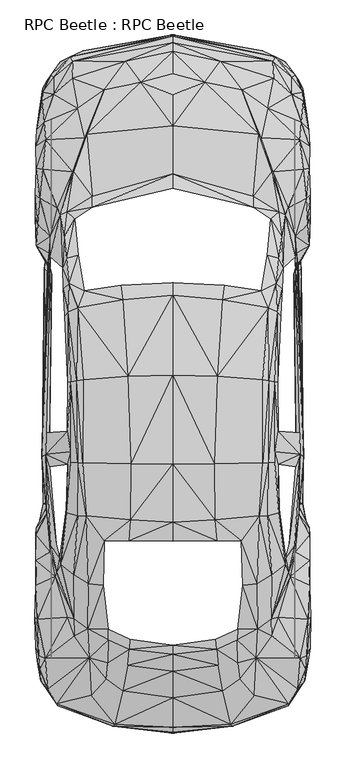
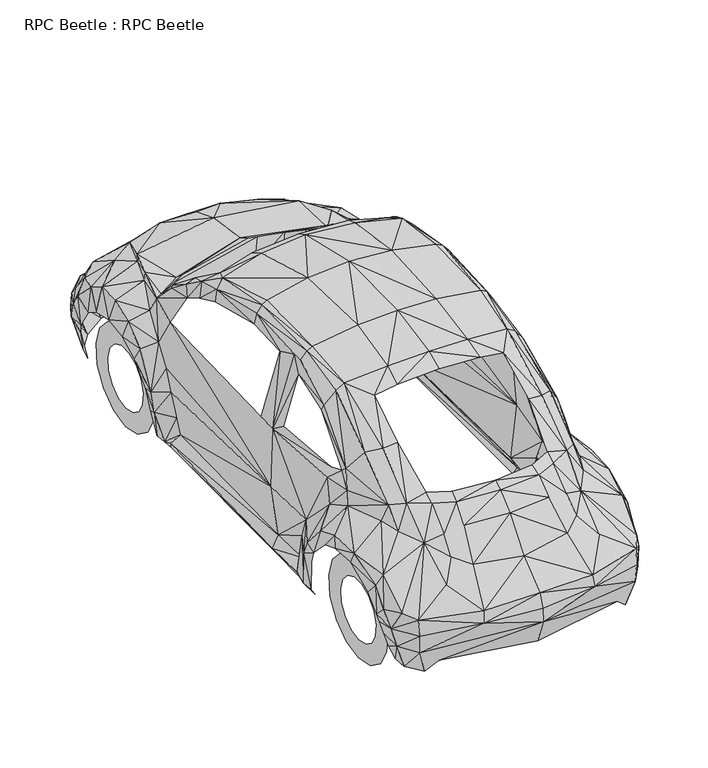
"""IFC4 building model written with IfcOpenShell, lengths in millimetres: proxy geometry, RPC Beetle : RPC Beetle."""

from ifc_helpers import new_model, si_unit, origin, place, context, project, spatial, triangles, source, transform, mapped, element, save


def rpc_beetle_rpc_beetle_31f8b51e(model_context):
    return source(origin(), model_context, "Body", "Tessellation", [
        triangles([(0.0, -748.5640469, 521.3894322), (0.0, -720.14536, 603.624202), (0.0, -696.6746996, 283.1362969), (0.0, -552.698168, 738.4051466), (0.0, -753.249444, 438.4540512), (0.0, -253.6666567, 1039.7136446), (0.0, -401.1024794, 921.3971746), (0.0, -304.8115909, 1012.258271), (0.0, 339.3169338, 1395.7139351), (0.0, 448.6129515, 1442.1297066), (0.0, 778.077507, 1504.0467121), (0.0, 1285.0167675, 1509.4764679), (0.0, 1741.0736687, 1402.3260315), (0.0, 2430.9612099, 967.1999022), (0.0, 3130.000518, 632.0428888), (0.0, 3001.4374352, 771.5092306), (0.0, 2704.2451103, 928.7536297), (0.0, 3164.1993027, 220.1684652), (0.0, 2883.1647125, 858.7358831), (0.0, 3222.5256844, 395.8040746), (0.0, 3178.9998528, 555.7633879), (0.0, 3213.9430687, 530.2784972), (-338.1784132, -715.5037828, 523.0096095), (-331.0409128, -702.1482754, 593.4652654), (-244.7338081, -218.0228295, 1034.0649342), (-248.9812959, -275.9549947, 1002.9312967), (-257.7389917, -368.17353, 911.8513184), (-249.0688632, 342.8199903, 1381.001025), (-285.238149, -511.5370176, 760.4306917), (-240.1360146, 460.0855433, 1426.5848705), (-236.4577871, 780.8799522, 1493.4060825), (-652.4921494, -590.2249108, 370.4943186), (-540.0870918, -593.333878, 283.4428189), (-181.240518, 2954.2772324, 806.3210592), (-253.1849819, 1278.5798058, 1496.1647804), (-379.8650402, -444.3655, 798.2639929), (-370.9321916, -353.3292326, 889.1688366), (-367.9983953, -222.2265337, 1003.4567734), (-368.3924847, -160.7037264, 1036.6922447), (-390.1553641, 342.863774, 1359.0192272), (-282.5670547, 1713.2680984, 1399.3047043), (-397.3366482, 87.4893818, 1215.3492176), (-463.1069432, -537.7663033, 704.8193333), (-271.4885704, 3072.331073, 662.6948696), (-475.7618394, -323.0714138, 849.8468182), (-463.7199872, 3085.9055351, 214.2570346), (-482.2425121, 95.7654028, 1203.3950054), (-485.0449937, -159.3024857, 1005.0769506), (-568.7247697, 3071.499147, 546.7429356), (-493.539933, 483.2496454, 1391.2913853), (-583.2625451, 3099.3922119, 522.0462599), (-510.267146, 3132.2774139, 369.399618), (-391.8631087, 2911.6272194, 782.7628315), (-656.3455479, -597.8441042, 480.0968946), (-660.2426937, -584.8389387, 576.2563957), (-562.2878443, -200.0695649, 879.7105476), (-560.0546594, -101.457906, 987.167506), (-512.4565836, 786.1783207, 1448.435281), (-541.7948364, 484.7822554, 1359.8511532), (-563.9956252, 148.5743069, 1172.305188), (-608.4846974, -561.2369273, 218.4607206), (-511.2742793, 1258.5246346, 1456.1858253), (-542.4078804, 784.6895308, 1430.657151), (-458.8594554, 2304.0621243, 949.0276829), (-601.0406751, -92.7440029, 893.1973698), (-503.7426533, 1765.2887604, 1320.9670441), (-546.0423243, 1253.0073841, 1441.5166626), (-603.011158, 501.1591264, 1278.5798058), (-580.1535416, 788.8932713, 1378.7239838), (-607.2148258, 519.8568223, 1235.1416142), (-601.2595934, 965.2732029, 1337.0374294), (-712.4823103, -503.0858256, 590.4876492), (-542.6706187, 1670.0487888, 1361.1648811), (-490.6061368, 2657.8732315, 893.5038918), (-599.6394161, 778.077507, 1307.3050873), (-598.0630589, 1243.7242298, 1343.7809132), (-639.5745512, 208.1266494, 1062.483621), (-680.4291796, -470.2006963, 218.6796571), (-538.4669146, 1966.7157097, 1180.581209), (-580.9855402, 1248.2344196, 1401.7567348), (-644.5226503, 243.2887836, 1028.2848364), (-502.3414307, 2635.8036484, 866.0047709), (-660.7243504, 162.2363182, 955.24569), (-690.2378105, -396.5922532, 226.8243271), (-559.1350934, 2175.0175301, 1011.1635704), (-670.1826393, 140.8675371, 872.7043619), (-662.475915, 324.2974654, 1009.4558258), (-615.0967575, 1623.4578827, 1262.1154037), (-594.6475333, 1646.0964718, 1321.2735661), (-589.4367322, 1809.6026253, 1269.4280388), (-728.8154703, -481.9797738, 373.2091965), (-751.5854467, -454.4368329, 476.550018), (-694.047389, 315.3208331, 957.7854332), (-726.5822491, -327.3188653, 735.5588814), (-622.9348692, 1777.2429726, 1192.7981958), (-564.6524529, 2445.7178673, 934.1396381), (-731.7930502, -393.8773753, 324.1223308), (-571.0017746, 2444.2728973, 884.1769901), (-698.6452188, 279.8521769, 807.6347145), (-604.2809933, 1949.769651, 1170.4660561), (-587.4224293, 3013.0852707, 200.1133485), (-690.9384218, 574.2421291, 283.6179717), (-750.2280441, -381.0035608, 396.9863425), (-627.532699, 1896.2601265, 1124.7070759), (-602.4856813, 2215.5656364, 949.1590702), (-619.4318127, 2072.8151928, 1075.2699045), (-710.4680437, 549.6329844, 448.6129515), (-764.7219995, -360.335382, 467.5296021), (-699.5209648, 762.6201656, 1015.4986256), (-763.3207769, -313.2189992, 670.9270706), (-757.8472012, -390.9435428, 564.6524529), (-717.4742294, 496.2986309, 583.5690671), (-722.7288506, 461.224064, 180.9777796), (-717.6493641, 554.4497326, 179.883079), (-771.4654106, -341.8128571, 511.011541), (-573.9356071, 2975.4709969, 682.6185808), (-730.7859169, 375.8802907, 185.1814838), (-541.1818288, 2805.3964943, 782.9380388), (-639.7496859, 2198.4444431, 944.2547911), (-738.9305506, 551.5596837, 222.4016865), (-781.5805635, -268.7736925, 609.2290924), (-772.2974092, -106.0556994, 755.9205019), (-721.7217173, 957.7416132, 967.0247675), (-703.3305433, 810.1306377, 292.3318839), (-724.8306845, 835.0462681, 964.3537096), (-757.7596338, 370.5381022, 225.46687), (-785.3463947, -89.9415395, 695.4924316), (-779.6538643, 80.9211054, 675.5686478), (-779.3911623, 89.5036484, 754.6506666), (-760.3869444, 444.1027617, 223.1460814), (-778.077507, 192.1000659, 630.9044409), (-658.6225164, 2237.1534176, 849.7592508), (-770.939934, 345.4910846, 426.1932807), (-774.1802885, 315.1456985, 501.684603), (-781.1864742, 232.2541011, 695.886521), (-719.225794, 810.0868904, 185.8383114), (-689.8874685, 1858.8647346, 293.9082775), (-696.6746996, 1958.8776707, 956.4279579), (-779.7414316, 377.369117, 532.3803311), (-778.1212543, 416.9976937, 439.7239228), (-745.498827, 819.5889267, 613.6517149), (-677.7143017, 2884.8288551, 670.6205486), (-697.5504456, 2077.4130226, 756.8838879), (-639.6182985, 3069.1783585, 391.6879377), (-713.0077869, 1918.2419243, 536.7153863), (-718.1748407, 1909.878336, 192.97583), (-705.1696753, 1981.9541691, 648.2884089), (-730.7859169, 1891.093, 233.3488017), (-673.9922905, 2907.8614609, 198.6683241), (-726.8887711, 2038.9229301, 189.9544301), (-721.6341499, 1973.3715534, 189.9544301), (-678.1959583, 2982.5647499, 540.5250011), (-699.6085321, 2815.6868546, 206.1999501), (-696.3681776, 2991.5851295, 517.4046827), (-723.6484165, 2624.6813622, 787.579616), (-699.0830555, 1882.4667824, 390.3742825), (-764.8971342, 2042.1632847, 362.5686032), (-741.7768158, 2457.6720795, 808.6856678), (-716.1605742, 2965.1367439, 449.5325174), (-766.4297441, 2001.1335217, 376.580902), (-731.5740955, 2724.4316689, 727.6331297), (-771.1588886, 2084.5942703, 482.2425121), (-759.1171091, 2291.4073734, 780.0917736), (-769.0132347, 2143.3146687, 699.0393082), (-777.5520304, 2022.8525448, 494.8098046), (-742.4774271, 2846.864312, 601.8726374), (-782.1060402, 2185.6581596, 616.4542328), (-739.5435946, 2918.4145958, 427.3755486), (-741.1200245, 2896.5202927, 519.8130386), (-750.4031788, 2804.433181, 398.0810795), (-782.2373549, 2313.1701439, 680.7357016), (-778.077507, 2462.7953133, 693.5219124), (-759.9052877, 2786.6113037, 455.2250115), (-774.1802885, 2682.8324638, 602.6608523), (-780.3544756, 2589.4317696, 666.3293135), (-742.6088144, 809.1235044, 220.3874199), (0.0, 2349.0768185, 1011.1635704), (-458.8594554, 2239.9558628, 1006.6095606), (0.0, 1812.0110538, 1368.2148869), (-293.9520611, 1795.8092812, 1359.1506145), (-580.2411452, 849.7154308, 1381.7892036), (338.1784132, -715.5037828, 523.0096095), (331.0409128, -702.1482754, 593.4652654), (244.7338081, -218.0228295, 1034.0649342), (248.9812959, -275.9549947, 1002.9312967), (257.7389917, -368.17353, 911.8513184), (249.0688632, 342.8199903, 1381.001025), (285.238149, -511.5370176, 760.4306917), (240.1360146, 460.0855433, 1426.5848705), (236.4577871, 780.8799522, 1493.4060825), (652.4921494, -590.2249108, 370.4943186), (540.0870918, -593.333878, 283.4428189), (181.240518, 2954.2772324, 806.3210592), (253.1849819, 1278.5798058, 1496.1647804), (379.8650402, -444.3655, 798.2639929), (370.9321916, -353.3292326, 889.1688366), (367.9983953, -222.2265337, 1003.4567734), (368.3924847, -160.7037264, 1036.6922447), (390.1553641, 342.863774, 1359.0192272), (282.5670547, 1713.2680984, 1399.3047043), (397.3366482, 87.4893818, 1215.3492176), (463.1069432, -537.7663033, 704.8193333), (271.4885704, 3072.331073, 662.6948696), (475.7618394, -323.0714138, 849.8468182), (463.7199872, 3085.9055351, 214.2570346), (482.2425121, 95.7654028, 1203.3950054), (485.0449937, -159.3024857, 1005.0769506), (568.7247697, 3071.499147, 546.7429356), (493.539933, 483.2496454, 1391.2913853), (583.2625451, 3099.3922119, 522.0462599), (510.267146, 3132.2774139, 369.399618), (391.8631087, 2911.6272194, 782.7628315), (656.3455479, -597.8441042, 480.0968946), (660.2426937, -584.8389387, 576.2563957), (562.2878443, -200.0695649, 879.7105476), (560.0546594, -101.457906, 987.167506), (512.4565836, 786.1783207, 1448.435281), (541.7948364, 484.7822554, 1359.8511532), (563.9956252, 148.5743069, 1172.305188), (608.4846974, -561.2369273, 218.4607206), (511.2742793, 1258.5246346, 1456.1858253), (542.4078804, 784.6895308, 1430.657151), (458.8594554, 2304.0621243, 949.0276829), (601.0406751, -92.7440029, 893.1973698), (503.7426533, 1765.2887604, 1320.9670441), (546.0423243, 1253.0073841, 1441.5166626), (603.011158, 501.1591264, 1278.5798058), (580.1535416, 788.8932713, 1378.7239838), (607.2148258, 519.8568223, 1235.1416142), (601.2595934, 965.2732029, 1337.0374294), (712.4823103, -503.0858256, 590.4876492), (542.6706187, 1670.0487888, 1361.1648811), (490.6061368, 2657.8732315, 893.5038918), (599.6394161, 778.077507, 1307.3050873), (598.0630589, 1243.7242298, 1343.7809132), (639.5745512, 208.1266494, 1062.483621), (680.4729996, -470.2006963, 218.6796571), (538.4669146, 1966.7157097, 1180.581209), (580.9855402, 1248.2344196, 1401.7567348), (644.5226503, 243.2887836, 1028.2848364), (502.3414307, 2635.8036484, 866.0047709), (660.7243504, 162.2363182, 955.24569), (690.2378105, -396.5922532, 226.8243271), (559.1350934, 2175.0175301, 1011.1635704), (670.1826393, 140.8675371, 872.7043619), (662.475915, 324.2974654, 1009.4558258), (615.0967575, 1623.4578827, 1262.1154037), (594.6475333, 1646.0964718, 1321.2735661), (589.4367322, 1809.6026253, 1269.4280388), (728.8154703, -481.9797738, 373.2091965), (751.5854467, -454.4368329, 476.550018), (694.047389, 315.3208331, 957.7854332), (726.5822491, -327.3188653, 735.5588814), (622.9348692, 1777.2429726, 1192.7981958), (564.6524529, 2445.7178673, 934.1396381), (731.7930502, -393.8773753, 324.1223308), (571.0017746, 2444.2728973, 884.1769901), (698.6452188, 279.8521769, 807.6347145), (604.2809933, 1949.769651, 1170.4660561), (587.4224293, 3013.0852707, 200.1133485), (690.9384218, 574.2421291, 283.6179717), (750.2280441, -381.0035608, 396.9863425), (627.532699, 1896.2601265, 1124.7070759), (602.4856813, 2215.5656364, 949.1590702), (619.4318127, 2072.8151928, 1075.2699045), (710.4680437, 549.6329844, 448.6129515), (764.7219995, -360.335382, 467.5296021), (699.5209648, 762.6201656, 1015.4986256), (763.3207769, -313.2189992, 670.9270706), (757.8472012, -390.9435428, 564.6524529), (717.4742294, 496.2986309, 583.5690671), (722.7288506, 461.224064, 180.9777796), (717.6493641, 554.4497326, 179.883079), (771.4654106, -341.8128571, 511.011541), (573.9356071, 2975.4709969, 682.6185808), (730.7859169, 375.8802907, 185.1814838), (541.1818288, 2805.3964943, 782.9380388), (639.7496859, 2198.4444431, 944.2547911), (738.9305506, 551.5596837, 222.4016865), (781.5805635, -268.7736925, 609.2290924), (772.2974092, -106.0556994, 755.9205019), (721.7654646, 957.7416132, 967.0247675), (703.3305433, 810.1306377, 292.3318839), (724.8306845, 835.0462681, 964.3537096), (757.7596338, 370.5381022, 225.46687), (785.3463947, -89.9415395, 695.4924316), (779.6538643, 80.9211054, 675.5686478), (779.4349096, 89.5036484, 754.6506666), (760.3869444, 444.1027617, 223.1460814), (778.077507, 192.1000659, 630.9044409), (658.6225164, 2237.1534176, 849.7592508), (770.939934, 345.4910846, 426.1932807), (774.1802885, 315.1456985, 501.684603), (781.1864742, 232.2541011, 695.886521), (719.225794, 810.0868904, 185.8383114), (689.8874685, 1858.8647346, 293.9082775), (696.6746996, 1958.8776707, 956.4279579), (779.7414316, 377.369117, 532.3803311), (778.1212543, 416.9976937, 439.7239228), (745.498827, 819.5889267, 613.6517149), (677.7143017, 2884.8288551, 670.6205486), (697.5504456, 2077.4130226, 756.8838879), (639.6182985, 3069.1783585, 391.6879377), (713.0077869, 1918.2419243, 536.7153863), (718.1748407, 1909.878336, 192.97583), (705.1696753, 1981.9541691, 648.2884089), (730.7859169, 1891.093, 233.3488017), (673.9922905, 2907.8614609, 198.6683241), (726.8887711, 2038.9229301, 189.9544301), (721.6341499, 1973.3715534, 189.9544301), (678.1959583, 2982.5647499, 540.5250011), (699.6085321, 2815.6868546, 206.1999501), (696.3681776, 2991.5851295, 517.4046827), (723.6484165, 2624.6813622, 787.579616), (699.0830555, 1882.4667824, 390.3742825), (764.8971342, 2042.1632847, 362.5686032), (741.7768158, 2457.6720795, 808.6856678), (716.1605742, 2965.1367439, 449.5325174), (766.4297441, 2001.1335217, 376.580902), (731.5740955, 2724.4316689, 727.6331297), (771.2027086, 2084.5942703, 482.2425121), (759.1171091, 2291.4073734, 780.0917736), (769.0132347, 2143.3146687, 699.0393082), (777.5520304, 2022.8525448, 494.8098046), (742.4774271, 2846.864312, 601.8726374), (782.1060402, 2185.6581596, 616.4542328), (739.5435946, 2918.4145958, 427.3755486), (741.1200245, 2896.5202927, 519.8130386), (750.4031788, 2804.433181, 398.0810795), (782.2373549, 2313.1701439, 680.7357016), (778.077507, 2462.7953133, 693.5219124), (759.9052877, 2786.6113037, 455.2250115), (774.1802885, 2682.8324638, 602.6608523), (780.3544756, 2589.4317696, 666.3293135), (742.6088144, 809.1235044, 220.3874199), (458.8594554, 2239.9558628, 1006.6095606), (293.9520611, 1795.8092812, 1359.1506145), (580.2411452, 849.7154308, 1381.7892036), (-693.1716431, 2430.2605259, 0.0015107), (-693.1716431, 2430.2605259, 117.8363121), (-693.1716431, 2557.1157188, 26.9752135), (-693.1716431, 2507.7661148, 134.3007777), (-693.1716431, 2661.9892593, 103.1671675), (-693.1716431, 2571.9162689, 180.8917202), (-693.1716431, 2726.8399521, 215.4846123), (-693.1716431, 2611.5449547, 249.552046), (-693.1716431, 2740.4144142, 344.4416937), (-693.1716431, 2619.820903, 328.3713083), (-693.1716431, 2700.3479645, 467.7938301), (-693.1716431, 2595.3430367, 403.7312797), (-693.1716431, 2613.5590759, 564.1285023), (-693.1716431, 2542.3151688, 462.6267763), (-693.1716431, 2495.111364, 616.8935955), (-693.1716431, 2469.8890663, 494.898898), (-693.1716431, 2365.4098331, 616.8935955), (-693.1716431, 2390.6319855, 494.898898), (-693.1716431, 2246.9619759, 564.1285023), (-693.1716431, 2318.205883, 462.6267763), (-693.1716431, 2160.1732327, 467.7938301), (-693.1716431, 2265.1780151, 403.7312797), (-693.1716431, 2120.1067829, 344.4416937), (-693.1716431, 2240.7002941, 328.3713083), (-693.1716431, 2133.681245, 215.4846123), (-693.1716431, 2248.9762424, 249.552046), (-693.1716431, 2198.5319378, 103.1671675), (-693.1716431, 2288.6049282, 180.8917202), (-693.1716431, 2303.4053329, 26.9752135), (-693.1716431, 2352.754937, 134.3007777), (693.1716431, 2430.2605259, 0.0015107), (693.1716431, 2430.2605259, 117.8363121), (693.1716431, 2303.4053329, 26.9752135), (693.1716431, 2352.754937, 134.3007777), (693.1716431, 2198.5319378, 103.1671675), (693.1716431, 2288.6049282, 180.8917202), (693.1716431, 2133.681245, 215.4846123), (693.1716431, 2248.9762424, 249.552046), (693.1716431, 2120.1067829, 344.4416937), (693.1716431, 2240.7002941, 328.3713083), (693.1716431, 2160.1732327, 467.7938301), (693.1716431, 2265.1780151, 403.7312797), (693.1716431, 2246.9619759, 564.1285023), (693.1716431, 2318.205883, 462.6267763), (693.1716431, 2365.4098331, 616.8935955), (693.1716431, 2390.6319855, 494.898898), (693.1716431, 2495.111364, 616.8935955), (693.1716431, 2469.8890663, 494.898898), (693.1716431, 2613.5590759, 564.1285023), (693.1716431, 2542.3151688, 462.6267763), (693.1716431, 2700.3479645, 467.7938301), (693.1716431, 2595.3430367, 403.7312797), (693.1716431, 2740.4144142, 344.4416937), (693.1716431, 2619.820903, 328.3713083), (693.1716431, 2726.8399521, 215.4846123), (693.1716431, 2611.5449547, 249.552046), (693.1716431, 2661.9892593, 103.1671675), (693.1716431, 2571.9162689, 180.8917202), (693.1716431, 2557.1157188, 26.9752135), (693.1716431, 2507.7661148, 134.3007777), (-693.1716431, -13.5744281, 0.0015107), (-693.1716431, -13.5744281, 117.8363121), (-693.1716431, 113.2807944, 26.9752135), (-693.1716431, 63.9311813, 134.3007777), (-693.1716431, 218.1541986, 103.1671675), (-693.1716431, 128.0812991, 180.8917202), (-693.1716431, 283.0049459, 215.4846123), (-693.1716431, 167.7098758, 249.552046), (-693.1716431, 296.5793717, 344.4416937), (-693.1716431, 175.9858968, 328.3713083), (-693.1716431, 256.5129038, 467.7938301), (-693.1716431, 151.5081395, 403.7312797), (-693.1716431, 169.7241424, 564.1285023), (-693.1716431, 98.4802897, 462.6267763), (-693.1716431, 51.2763078, 616.8935955), (-693.1716431, 26.0541442, 494.898898), (-693.1716431, -78.425164, 616.8935955), (-693.1716431, -53.2030025, 494.898898), (-693.1716431, -196.872994, 564.1285023), (-693.1716431, -125.6291504, 462.6267763), (-693.1716431, -283.6617735, 467.7938301), (-693.1716431, -178.6569911, 403.7312797), (-693.1716431, -323.7282414, 344.4416937), (-693.1716431, -203.1347484, 328.3713083), (-693.1716431, -310.1537793, 215.4846123), (-693.1716431, -194.8587274, 249.552046), (-693.1716431, -245.3030684, 103.1671675), (-693.1716431, -155.2301507, 180.8917202), (-693.1716431, -140.4296551, 26.9752135), (-693.1716431, -91.0800329, 134.3007777), (693.1716431, -13.5744281, 0.0015107), (693.1716431, -13.5744281, 117.8363121), (693.1716431, -140.4296551, 26.9752135), (693.1716431, -91.0800329, 134.3007777), (693.1716431, -245.3030684, 103.1671675), (693.1716431, -155.2301507, 180.8917202), (693.1716431, -310.1537793, 215.4846123), (693.1716431, -194.8587274, 249.552046), (693.1716431, -323.7282414, 344.4416937), (693.1716431, -203.1347484, 328.3713083), (693.1716431, -283.6617735, 467.7938301), (693.1716431, -178.6569911, 403.7312797), (693.1716431, -196.872994, 564.1285023), (693.1716431, -125.6291504, 462.6267763), (693.1716431, -78.425164, 616.8935955), (693.1716431, -53.2030025, 494.898898), (693.1716431, 51.2763078, 616.8935955), (693.1716431, 26.0541442, 494.898898), (693.1716431, 169.7241424, 564.1285023), (693.1716431, 98.4802897, 462.6267763), (693.1716431, 256.5129038, 467.7938301), (693.1716431, 151.5081395, 403.7312797), (693.1716431, 296.5793717, 344.4416937), (693.1716431, 175.9858968, 328.3713083), (693.1716431, 283.0049459, 215.4846123), (693.1716431, 167.7098758, 249.552046), (693.1716431, 218.1541986, 103.1671675), (693.1716431, 128.0812991, 180.8917202), (693.1716431, 113.2807944, 26.9752135), (693.1716431, 63.9311813, 134.3007777)], [[67, 58, 62], [67, 63, 58], [53, 82, 74], [34, 17, 19], [118, 82, 53], [155, 98, 82], [155, 158, 98], [34, 74, 17], [172, 155, 175], [172, 158, 155], [159, 168, 169], [166, 142, 169], [175, 161, 174], [175, 155, 161], [142, 152, 169], [154, 169, 152], [160, 145, 165], [160, 156, 145], [162, 160, 165], [162, 157, 160], [34, 53, 74], [74, 96, 64], [82, 96, 74], [82, 98, 96], [36, 29, 27], [29, 43, 24], [23, 55, 54], [23, 24, 55], [23, 2, 24], [23, 1, 2], [5, 1, 23], [134, 140, 133], [134, 139, 140], [117, 130, 113], [117, 126, 130], [113, 120, 114], [113, 130, 120], [140, 112, 107], [140, 139, 112], [92, 108, 103], [91, 103, 97], [91, 92, 103], [61, 33, 32], [84, 78, 91], [84, 91, 97], [38, 26, 25], [77, 81, 83], [63, 50, 58], [63, 59, 50], [68, 63, 69], [68, 59, 63], [181, 75, 69], [74, 64, 17], [64, 14, 17], [64, 178, 14], [178, 177, 14], [34, 19, 16], [53, 34, 44], [21, 44, 15], [21, 49, 44], [44, 34, 15], [34, 16, 15], [22, 49, 21], [22, 51, 49], [20, 51, 22], [20, 52, 51], [18, 52, 20], [18, 46, 52], [51, 152, 49], [51, 154, 152], [101, 144, 46], [144, 52, 46], [101, 159, 144], [159, 169, 154], [101, 168, 159], [101, 149, 168], [149, 170, 168], [149, 153, 170], [168, 173, 169], [168, 170, 173], [49, 142, 116], [49, 152, 142], [49, 116, 44], [116, 142, 118], [161, 155, 118], [155, 82, 118], [142, 161, 118], [158, 132, 98], [158, 163, 132], [172, 163, 158], [172, 171, 163], [98, 119, 96], [98, 132, 119], [171, 164, 163], [171, 167, 164], [163, 143, 132], [163, 164, 143], [96, 105, 64], [96, 119, 105], [105, 178, 64], [105, 85, 178], [167, 165, 164], [167, 162, 165], [165, 143, 164], [165, 147, 143], [150, 160, 157], [150, 151, 160], [151, 156, 160], [151, 148, 137], [13, 35, 12], [13, 41, 35], [12, 31, 11], [12, 35, 31], [35, 58, 31], [35, 62, 58], [11, 30, 10], [11, 31, 30], [31, 50, 30], [31, 58, 50], [10, 28, 9], [10, 30, 28], [30, 40, 28], [30, 50, 40], [125, 75, 181], [125, 109, 75], [125, 87, 109], [125, 93, 87], [123, 141, 125], [137, 141, 156], [137, 124, 141], [148, 124, 137], [148, 176, 124], [146, 176, 148], [146, 136, 176], [141, 112, 125], [112, 93, 125], [112, 99, 93], [124, 112, 141], [124, 107, 112], [124, 102, 107], [176, 102, 124], [176, 120, 102], [136, 120, 176], [136, 114, 120], [47, 40, 50], [47, 42, 40], [48, 42, 47], [48, 39, 42], [57, 47, 60], [57, 48, 47], [60, 50, 59], [60, 47, 50], [59, 77, 60], [59, 68, 77], [77, 57, 60], [77, 83, 57], [70, 77, 68], [70, 81, 77], [75, 68, 69], [75, 70, 68], [26, 6, 25], [26, 8, 6], [27, 8, 26], [27, 7, 8], [29, 7, 27], [29, 4, 7], [24, 4, 29], [24, 2, 4], [32, 5, 23], [33, 5, 32], [33, 3, 5], [32, 23, 54], [55, 45, 72], [55, 24, 43], [99, 83, 93], [99, 86, 83], [135, 86, 99], [135, 129, 86], [131, 129, 135], [131, 128, 129], [93, 81, 87], [93, 83, 81], [128, 122, 129], [128, 127, 122], [122, 86, 129], [122, 65, 86], [86, 57, 83], [86, 65, 57], [127, 110, 122], [127, 121, 110], [110, 94, 122], [122, 94, 65], [94, 56, 65], [56, 57, 65], [56, 48, 57], [56, 45, 48], [94, 45, 56], [115, 110, 121], [115, 111, 110], [111, 94, 110], [111, 72, 94], [108, 92, 115], [92, 111, 115], [78, 32, 91], [78, 61, 32], [45, 38, 48], [45, 37, 38], [37, 26, 38], [37, 27, 26], [36, 27, 37], [134, 135, 139], [134, 131, 135], [139, 99, 112], [139, 135, 99], [126, 140, 130], [126, 133, 140], [130, 107, 120], [130, 140, 107], [120, 107, 102], [45, 36, 37], [92, 55, 72], [92, 54, 55], [91, 54, 92], [91, 32, 54], [92, 72, 111], [72, 45, 94], [43, 45, 55], [43, 36, 45], [43, 29, 36], [79, 90, 66], [79, 100, 90], [90, 73, 66], [85, 100, 79], [85, 106, 100], [85, 105, 106], [105, 119, 106], [95, 88, 89], [90, 89, 73], [89, 67, 73], [73, 67, 62], [89, 76, 80], [89, 80, 67], [88, 76, 89], [73, 35, 41], [73, 62, 35], [69, 63, 181], [80, 63, 67], [76, 71, 80], [146, 148, 151], [141, 147, 145], [151, 137, 156], [173, 166, 169], [173, 174, 166], [166, 174, 161], [166, 161, 142], [52, 144, 51], [144, 154, 51], [144, 159, 154], [116, 53, 44], [116, 118, 53], [119, 143, 138], [143, 119, 132], [143, 147, 138], [138, 104, 119], [119, 104, 106], [104, 100, 106], [104, 90, 100], [104, 95, 90], [95, 89, 90], [25, 39, 38], [38, 39, 48], [141, 138, 147], [156, 141, 145], [165, 145, 147], [41, 179, 180], [41, 13, 179], [66, 41, 180], [66, 73, 41], [123, 125, 71], [125, 181, 71], [71, 181, 80], [181, 63, 80], [138, 141, 123], [226, 221, 217], [226, 217, 222], [212, 233, 241], [193, 19, 17], [277, 212, 241], [314, 241, 257], [314, 257, 317], [193, 17, 233], [331, 334, 314], [331, 314, 317], [318, 328, 327], [325, 328, 301], [334, 333, 320], [334, 320, 314], [301, 328, 311], [313, 311, 328], [319, 324, 304], [319, 304, 315], [321, 324, 319], [321, 319, 316], [193, 233, 212], [233, 223, 255], [241, 233, 255], [241, 255, 257], [195, 186, 188], [188, 183, 202], [182, 213, 214], [182, 214, 183], [182, 183, 2], [182, 2, 1], [5, 182, 1], [293, 292, 299], [293, 299, 298], [276, 272, 289], [276, 289, 285], [272, 273, 279], [272, 279, 289], [299, 266, 271], [299, 271, 298], [251, 262, 267], [250, 256, 262], [250, 262, 251], [220, 191, 192], [243, 250, 237], [243, 256, 250], [197, 184, 185], [236, 242, 240], [222, 217, 209], [222, 209, 218], [227, 228, 222], [227, 222, 218], [338, 228, 234], [233, 17, 223], [223, 17, 14], [223, 14, 336], [336, 14, 177], [193, 16, 19], [212, 203, 193], [21, 15, 203], [21, 203, 208], [203, 15, 193], [193, 15, 16], [22, 21, 208], [22, 208, 210], [20, 22, 210], [20, 210, 211], [18, 20, 211], [18, 211, 205], [210, 208, 311], [210, 311, 313], [260, 205, 303], [303, 205, 211], [260, 303, 318], [318, 313, 328], [260, 318, 327], [260, 327, 308], [308, 327, 329], [308, 329, 312], [327, 328, 332], [327, 332, 329], [208, 275, 301], [208, 301, 311], [208, 203, 275], [275, 277, 301], [320, 277, 314], [314, 277, 241], [301, 277, 320], [317, 257, 291], [317, 291, 322], [331, 317, 322], [331, 322, 330], [257, 255, 278], [257, 278, 291], [330, 322, 323], [330, 323, 326], [322, 291, 302], [322, 302, 323], [255, 223, 264], [255, 264, 278], [264, 223, 336], [264, 336, 244], [326, 323, 324], [326, 324, 321], [324, 323, 302], [324, 302, 306], [309, 316, 319], [309, 319, 310], [310, 319, 315], [310, 296, 307], [13, 12, 194], [13, 194, 200], [12, 11, 190], [12, 190, 194], [194, 190, 217], [194, 217, 221], [11, 10, 189], [11, 189, 190], [190, 189, 209], [190, 209, 217], [10, 9, 187], [10, 187, 189], [189, 187, 199], [189, 199, 209], [284, 338, 234], [284, 234, 268], [284, 268, 246], [284, 246, 252], [282, 284, 300], [296, 315, 300], [296, 300, 283], [307, 296, 283], [307, 283, 335], [305, 307, 335], [305, 335, 295], [300, 284, 271], [271, 284, 252], [271, 252, 258], [283, 300, 271], [283, 271, 266], [283, 266, 261], [335, 283, 261], [335, 261, 279], [295, 335, 279], [295, 279, 273], [206, 209, 199], [206, 199, 201], [207, 206, 201], [207, 201, 198], [216, 219, 206], [216, 206, 207], [219, 218, 209], [219, 209, 206], [218, 219, 236], [218, 236, 227], [236, 219, 216], [236, 216, 242], [229, 227, 236], [229, 236, 240], [234, 228, 227], [234, 227, 229], [185, 184, 6], [185, 6, 8], [186, 185, 8], [186, 8, 7], [188, 186, 7], [188, 7, 4], [183, 188, 4], [183, 4, 2], [191, 182, 5], [192, 191, 5], [192, 5, 3], [191, 213, 182], [214, 231, 204], [214, 202, 183], [258, 252, 242], [258, 242, 245], [294, 258, 245], [294, 245, 288], [290, 294, 288], [290, 288, 287], [252, 246, 240], [252, 240, 242], [287, 288, 281], [287, 281, 286], [281, 288, 245], [281, 245, 224], [245, 242, 216], [245, 216, 224], [286, 281, 269], [286, 269, 280], [269, 281, 253], [281, 224, 253], [253, 224, 215], [215, 224, 216], [215, 216, 207], [215, 207, 204], [253, 215, 204], [274, 280, 269], [274, 269, 270], [270, 269, 253], [270, 253, 231], [267, 274, 251], [251, 274, 270], [237, 250, 191], [237, 191, 220], [204, 207, 197], [204, 197, 196], [196, 197, 185], [196, 185, 186], [195, 196, 186], [293, 298, 294], [293, 294, 290], [298, 271, 258], [298, 258, 294], [285, 289, 299], [285, 299, 292], [289, 279, 266], [289, 266, 299], [279, 261, 266], [204, 196, 195], [251, 231, 214], [251, 214, 213], [250, 251, 213], [250, 213, 191], [251, 270, 231], [231, 253, 204], [202, 214, 204], [202, 204, 195], [202, 195, 188], [238, 225, 249], [238, 249, 259], [249, 225, 232], [244, 238, 259], [244, 259, 265], [244, 265, 264], [264, 265, 278], [254, 248, 247], [249, 232, 248], [248, 232, 226], [232, 221, 226], [248, 239, 235], [248, 226, 239], [247, 248, 235], [232, 200, 194], [232, 194, 221], [228, 338, 222], [239, 226, 222], [235, 239, 230], [305, 310, 307], [300, 304, 306], [310, 315, 296], [332, 328, 325], [332, 325, 333], [325, 320, 333], [325, 301, 320], [211, 210, 303], [303, 210, 313], [303, 313, 318], [275, 203, 212], [275, 212, 277], [278, 297, 302], [302, 291, 278], [302, 297, 306], [297, 278, 263], [278, 265, 263], [263, 265, 259], [263, 259, 249], [263, 249, 254], [254, 249, 248], [184, 197, 198], [197, 207, 198], [300, 306, 297], [315, 304, 300], [324, 306, 304], [200, 337, 179], [200, 179, 13], [225, 337, 200], [225, 200, 232], [282, 230, 284], [284, 230, 338], [230, 239, 338], [338, 239, 222], [297, 282, 300], [339, 342, 341], [339, 340, 342], [341, 344, 343], [341, 342, 344], [343, 346, 345], [343, 344, 346], [345, 348, 347], [345, 346, 348], [347, 350, 349], [347, 348, 350], [349, 352, 351], [349, 350, 352], [351, 354, 353], [351, 352, 354], [353, 356, 355], [353, 354, 356], [355, 358, 357], [355, 356, 358], [357, 360, 359], [357, 358, 360], [359, 362, 361], [359, 360, 362], [361, 364, 363], [361, 362, 364], [363, 366, 365], [363, 364, 366], [365, 368, 367], [365, 366, 368], [367, 340, 339], [367, 368, 340], [369, 372, 371], [369, 370, 372], [371, 374, 373], [371, 372, 374], [373, 376, 375], [373, 374, 376], [375, 378, 377], [375, 376, 378], [377, 380, 379], [377, 378, 380], [379, 382, 381], [379, 380, 382], [381, 384, 383], [381, 382, 384], [383, 386, 385], [383, 384, 386], [385, 388, 387], [385, 386, 388], [387, 390, 389], [387, 388, 390], [389, 392, 391], [389, 390, 392], [391, 394, 393], [391, 392, 394], [393, 396, 395], [393, 394, 396], [395, 398, 397], [395, 396, 398], [397, 370, 369], [397, 398, 370], [399, 402, 401], [399, 400, 402], [401, 404, 403], [401, 402, 404], [403, 406, 405], [403, 404, 406], [405, 408, 407], [405, 406, 408], [407, 410, 409], [407, 408, 410], [409, 412, 411], [409, 410, 412], [411, 414, 413], [411, 412, 414], [413, 416, 415], [413, 414, 416], [415, 418, 417], [415, 416, 418], [417, 420, 419], [417, 418, 420], [419, 422, 421], [419, 420, 422], [421, 424, 423], [421, 422, 424], [423, 426, 425], [423, 424, 426], [425, 428, 427], [425, 426, 428], [427, 400, 399], [427, 428, 400], [429, 432, 431], [429, 430, 432], [431, 434, 433], [431, 432, 434], [433, 436, 435], [433, 434, 436], [435, 438, 437], [435, 436, 438], [437, 440, 439], [437, 438, 440], [439, 442, 441], [439, 440, 442], [441, 444, 443], [441, 442, 444], [443, 446, 445], [443, 444, 446], [445, 448, 447], [445, 446, 448], [447, 450, 449], [447, 448, 450], [449, 452, 451], [449, 450, 452], [451, 454, 453], [451, 452, 454], [453, 456, 455], [453, 454, 456], [455, 458, 457], [455, 456, 458], [457, 430, 429], [457, 458, 430]], closed=False),
    ])


if __name__ == "__main__":
    model = new_model("IFC4")
    model_context = context("Model", 3, world=origin())
    ifc_project = project(units=[si_unit("LENGTHUNIT", "METRE", prefix="MILLI")], contexts=[model_context])
    site = spatial("IfcSite", under=ifc_project)
    building = spatial("IfcBuilding", under=site)
    placement = place(None, origin())
    rpc_beetle_rpc_beetle_shape = rpc_beetle_rpc_beetle_31f8b51e(model_context)
    element("IfcBuildingElementProxy", 1, Name="RPC Beetle : RPC Beetle", ObjectType="RPC Beetle : RPC Beetle", at=placement, inside=building, context=model_context, shape_type="MappedRepresentation", body=[
        mapped(rpc_beetle_rpc_beetle_shape, transform((0.0, 0.0, 0.0), x_axis=(1.0, 0.0, 0.0), y_axis=(0.0, 1.0, 0.0), z_axis=(0.0, 0.0, 1.0))),
    ])
    save(model, "model.ifc")

# Revit data of these elements
# Type "RPC Beetle : RPC Beetle"
#   built-in parameter 1005198 = "{2, 15},{39, RPC-16-0U6E-L4EG-ENH1-J3KF-SVEL-0TX4-C0},{1, 0},{1, 0},{2, 36},{1, 8},{5, Color},{1, 0},{1, 0},{3, 0.8},{3, 0.8},{3, 0.8},{1, 8},{7, BBoxMin},{1, 0},{1, 0},{1, 0},{1, 0},{1, 0},{1, 8},{7, BBoxMax},{1, 0},{1, 0},{1, 0},{1, 0},{1, 0},{2, 11},{9, RPCTypeId},{1, 0},{1, 0},{39, RPC-16-0U6E-L4EG-ENH1-J3KF-SVEL-0TX4-C0},{1, 6},{14, RPCPlantHeight},{1, 0},{1, 0},{7, 4.91667},{2, 11},{20, AdvancedUIDefinition},{1, 0},{1, 0},{0, },{2, 11},{10, AssetLibID},{1, 0},{1, 0},{36, 4D3F6E72-3F99-4203-98E9-AF80B3C7A7A4},{2, 11},{10, BaseSchema},{1, 0},{1, 0},{9, RPCSchema},{2, 11},{12, ExchangeGUID},{1, 0},{1, 0},{0, },{1, 2},{6, Hidden},{1, 0},{1, 0},{1, 0},{2, 11},{12, LocalizedUID},{1, 0},{1, 0},{0, },{1, 4},{11, RPCCategory},{1, 0},{1, 0},{1, 0},{2, 11},{8, RPCImage},{1, 0},{1, 0},{0, },{1, 4},{13, SchemaVersion},{1, 0},{1, 0},{1, 4},{2, 11},{12, UIDefinition},{1, 0},{1, 0},{0, },{2, 11},{6, UIName},{1, 0},{1, 0},{39, RPC-16-0U6E-L4EG-ENH1-J3KF-SVEL-0TX4-C0},{2, 11},{11, VersionGUID},{1, 0},{1, 0},{9, RPCSchema},{2, 11},{9, assettype},{1, 0},{1, 0},{11, RPCGeometry},{2, 11},{11, description},{1, 0},{1, 0},{0, },{2, 11},{9, localname},{1, 0},{1, 0},{3, RPC},{2, 11},{9, localtype},{1, 0},{1, 0},{3, RPC},{1, 4},{8, revision},{1, 0},{1, 0},{1, 1},{2, 11},{9, thumbnail},{1, 0},{1, 0},{0, },{1, 4},{7, version},{1, 0},{1, 0},{1, 1},{2, 14},{6, Height},{1, 0},{1, 0},{7, 4.91667},{1, 2},{20, RPC_Cast Reflections},{1, 0},{1, 0},{1, 1},{1, 4},{16, RPC_Transparency},{1, 0},{1, 0},{2, 18},{1, 4},{11, RPC_Tinting},{1, 0},{1, 0},{2, 50},{1, 2},{15, RPC_Use Tinting},{1, 0},{1, 0},{1, 0},{1, 2},{17, RPC_License Plate},{1, 0},{1, 0},{1, 0},{2, 11},{25, RPC_License Plate Texture},{1, 0},{1, 0},{64, __RPC:/object data/textures/car/plate/textures/default/rgb/0/0/0},{2, 11},{27, RPC_i_License Plate Texture},{1, 0},{1, 0},{0, },{1, 2},{16, RPC_Custom Plate},{1, 0},{1, 0},{1, 0},{2, 11},{27, RPC_License Plate File Name},{1, 0},{1, 0},{0, },{2, 11},{7, keyword},{1, 0},{1, 0},{27, :Geometry:RPC:VW Beetle [4]},{2, 11},{8, category},{1, 0},{1, 0},{21, :Auto_Economy/Midsize},{21, assetlibrary_base.fbx},{1, 5},"
#   built-in parameter 1005195 = "RPC-16-0U6E-L4EG-ENH1-J3KF-SVEL-0TX4-C0"
#   Height = 0
